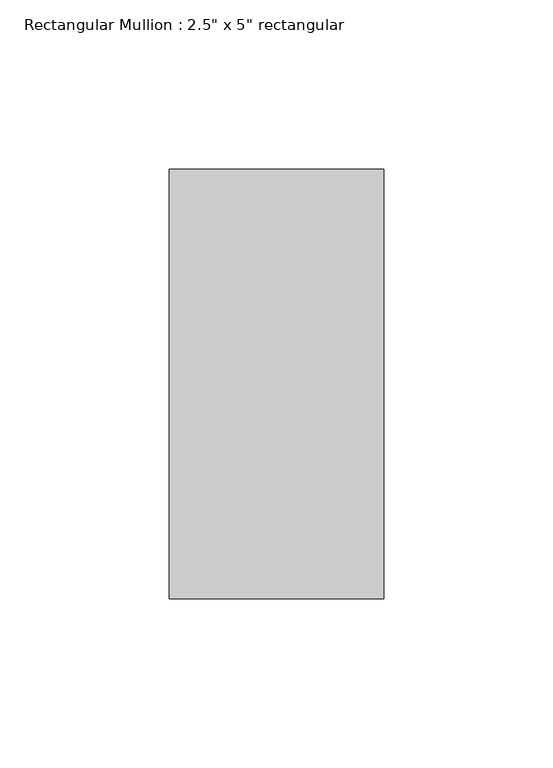
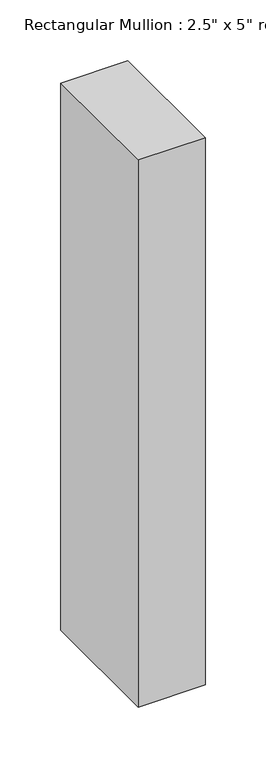
"""IFC4 building model written with IfcOpenShell, lengths in millimetres: member geometry."""

from ifc_helpers import new_model, si_unit, frame, origin, place, context, project, spatial, polyline, outline, extrude, source, transform, mapped, element, save


def member_61d667c8(model_context):
    return source(origin(), model_context, "Body", "SweptSolid", [
        extrude(outline(polyline([(0.0, 63.5), (0.0, -63.5), (-63.5, -63.5), (-63.5, 63.5), (0.0, 63.5)])), frame((0.0, 0.0, -549.036674), z_axis=(0.0, 0.0, 1.0), x_axis=(1.0, 0.0, 0.0)), (0.0, 0.0, 1.0), 549.036674),
    ])


if __name__ == "__main__":
    model = new_model("IFC4")
    model_context = context("Model", 3, world=origin())
    ifc_project = project(units=[si_unit("LENGTHUNIT", "METRE", prefix="MILLI")], contexts=[model_context])
    site = spatial("IfcSite", under=ifc_project)
    building = spatial("IfcBuilding", under=site)
    placement = place(None, origin())
    member_shape = member_61d667c8(model_context)
    element("IfcMember", 1, ObjectType="Rectangular Mullion : 2.5\" x 5\" rectangular", at=placement, inside=building, context=model_context, shape_type="MappedRepresentation", body=[
        mapped(member_shape, transform((0.0, 0.0, 0.0), x_axis=(1.0, 0.0, 0.0), y_axis=(0.0, 1.0, 0.0), z_axis=(0.0, 0.0, 1.0))),
    ])
    save(model, "model.ifc")

# Revit data of these elements
# Type "Rectangular Mullion : 2.5\" x 5\" rectangular"
#   built-in parameter 1007304 = 0.416667 (stored number, unit not read)
#   built-in parameter 1007301 = 0.104167 (stored number, unit not read)
#   built-in parameter 1007300 = 0.104167 (stored number, unit not read)
# Element 1 (IfcMember, "Rectangular Mullion : 2.5\" x 5\" rectangular")
#   Materials on its faces: "Aluminum"
# Materials
#   "Aluminum": class "Metal", colour RGB 247 247 247, transparency 0, Description = "Aluminum 6061", Cost = 0
